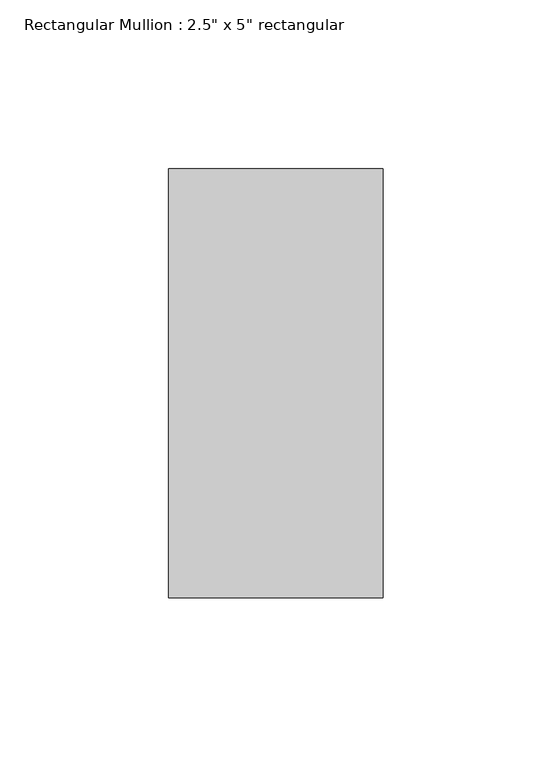
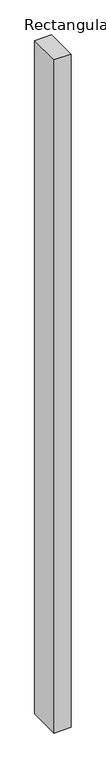
"""IFC4 building model written with IfcOpenShell, lengths in millimetres: member geometry."""

from ifc_helpers import new_model, si_unit, frame, origin, place, context, project, spatial, polyline, outline, extrude, source, transform, mapped, element, save


def member_6ba65f20(model_context):
    return source(origin(), model_context, "Body", "SweptSolid", [
        extrude(outline(polyline([(0.0, 63.5), (0.0, -63.5), (-63.5, -63.5), (-63.5, 63.5), (0.0, 63.5)])), frame((0.0, 0.0, -2667.0), z_axis=(0.0, 0.0, 1.0), x_axis=(1.0, 0.0, 0.0)), (0.0, 0.0, 1.0), 2667.0),
    ])


if __name__ == "__main__":
    model = new_model("IFC4")
    model_context = context("Model", 3, world=origin())
    ifc_project = project(units=[si_unit("LENGTHUNIT", "METRE", prefix="MILLI")], contexts=[model_context])
    site = spatial("IfcSite", under=ifc_project)
    building = spatial("IfcBuilding", under=site)
    placement = place(None, origin())
    member_shape = member_6ba65f20(model_context)
    element("IfcMember", 1, ObjectType="Rectangular Mullion : 2.5\" x 5\" rectangular", at=placement, inside=building, context=model_context, shape_type="MappedRepresentation", body=[
        mapped(member_shape, transform((0.0, 0.0, 0.0), x_axis=(1.0, 0.0, 0.0), y_axis=(0.0, 1.0, 0.0), z_axis=(0.0, 0.0, 1.0))),
    ])
    save(model, "model.ifc")

# Revit data of these elements
# Type "Rectangular Mullion : 2.5\" x 5\" rectangular"
#   built-in parameter 1007304 = 0.416667 (stored number, unit not read)
#   built-in parameter 1007301 = 0.104167 (stored number, unit not read)
#   built-in parameter 1007300 = 0.104167 (stored number, unit not read)
